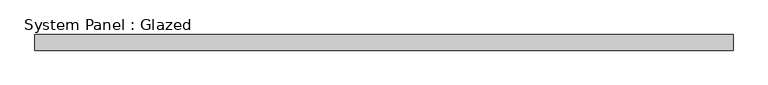
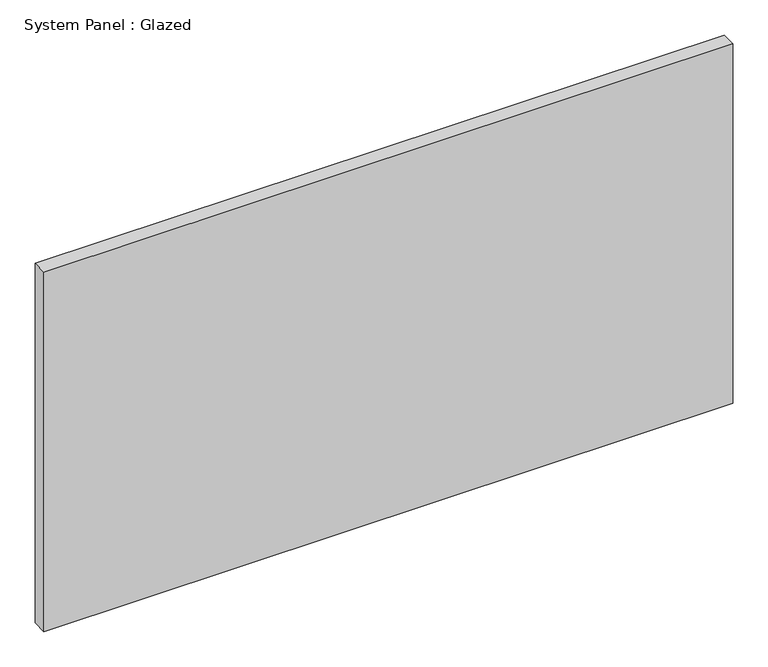
"""IFC4 building model written with IfcOpenShell, lengths in millimetres: plate geometry, System Panel : Glazed."""

from ifc_helpers import new_model, si_unit, origin, origin_with_axes, place, context, project, spatial, polyline, outline, extrude, source, transform, mapped, element, save


def system_panel_glazed_69f0b79b(model_context):
    return source(origin(), model_context, "Body", "SweptSolid", [
        extrude(outline(polyline([(568.3085922, 19.05), (-568.3085922, 19.05), (-568.3085922, 44.45), (568.3085922, 44.45), (568.3085922, 19.05)])), origin_with_axes(), (0.0, 0.0, 1.0), 627.1281505),
    ])


if __name__ == "__main__":
    model = new_model("IFC4")
    model_context = context("Model", 3, world=origin())
    ifc_project = project(units=[si_unit("LENGTHUNIT", "METRE", prefix="MILLI")], contexts=[model_context])
    site = spatial("IfcSite", under=ifc_project)
    building = spatial("IfcBuilding", under=site)
    placement = place(None, origin())
    system_panel_glazed_shape = system_panel_glazed_69f0b79b(model_context)
    element("IfcPlate", 1, ObjectType="System Panel : Glazed", at=placement, inside=building, context=model_context, shape_type="MappedRepresentation", body=[
        mapped(system_panel_glazed_shape, transform((0.0, 0.0, 0.0), x_axis=(1.0, 0.0, 0.0), y_axis=(0.0, 1.0, 0.0), z_axis=(0.0, 0.0, 1.0))),
    ])
    save(model, "model.ifc")

# Revit data of these elements
# Type "System Panel : Glazed"
#   Construction Type Id = "GSP4R"
#   Analytic Construction = "1/8 in Pilkington single glazing"
#   Visual Light Transmittance = 0.9
#   Solar Heat Gain Coefficient = 0.86
#   Heat Transfer Coefficient (U) = 1.18115 BTU/(h·ft²·°F)
#   Define Thermal Properties by = 1
# Element 1 (IfcPlate, "System Panel : Glazed")
#   Materials on its faces: "Glass"
# Materials
#   "Glass": class "Glass", colour RGB 0 128 192, transparency 0.75, Description = "Soda Lime Glass", Cost = 0
